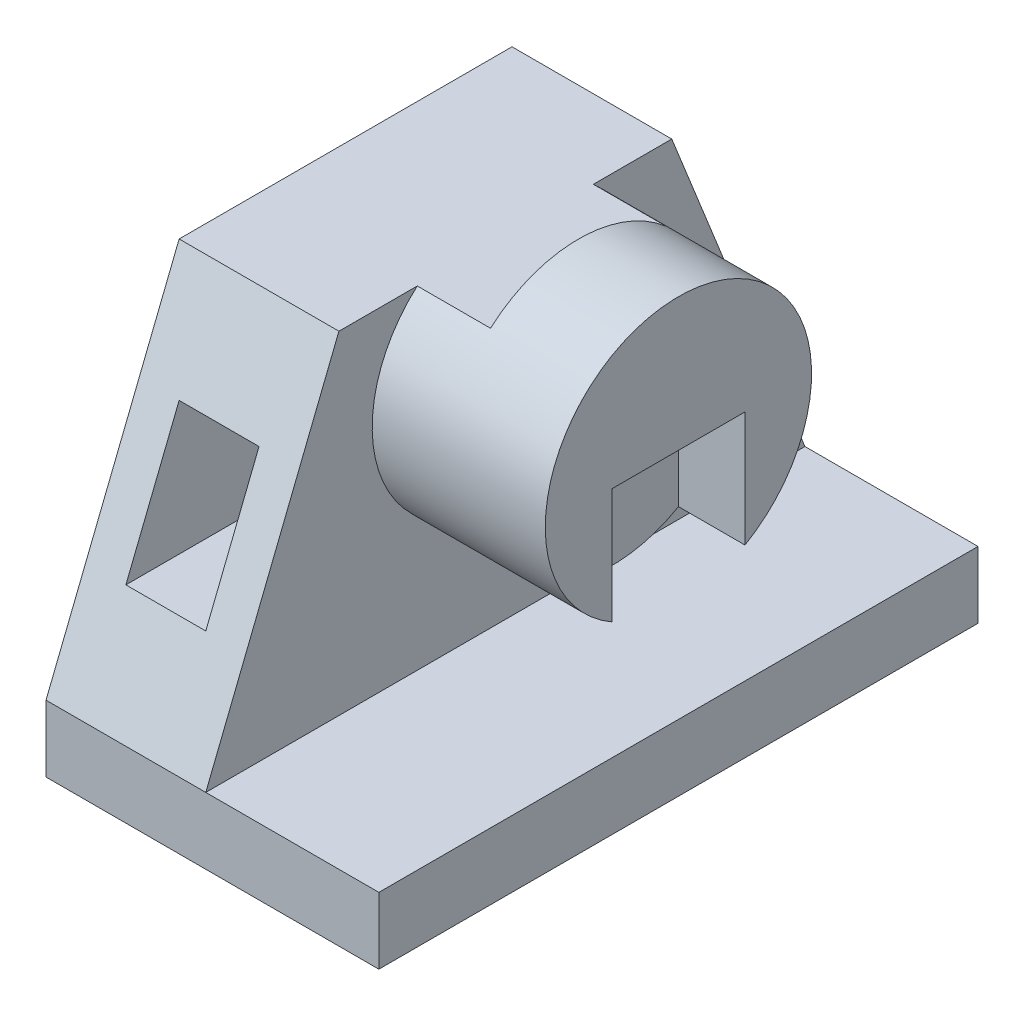
ISO-10303-21;
HEADER;
FILE_DESCRIPTION(('STEP AP214'),'2;1');
FILE_NAME('part.step','',(''),(''),'','','');
FILE_SCHEMA(('AUTOMOTIVE_DESIGN { 1 0 10303 214 1 1 1 1 }'));
ENDSEC;
DATA;
#1=APPLICATION_CONTEXT('core data for automotive mechanical design processes');
#2=APPLICATION_PROTOCOL_DEFINITION('international standard','automotive_design',2000,#1);
#3=PRODUCT_CONTEXT('',#1,'mechanical');
#4=PRODUCT('Part','Part','',(#3));
#5=PRODUCT_RELATED_PRODUCT_CATEGORY('part','',(#4));
#6=PRODUCT_DEFINITION_FORMATION('','',#4);
#7=PRODUCT_DEFINITION_CONTEXT('part definition',#1,'design');
#8=PRODUCT_DEFINITION('design','',#6,#7);
#9=PRODUCT_DEFINITION_SHAPE('','',#8);
#10=(LENGTH_UNIT() NAMED_UNIT(*) SI_UNIT(.MILLI.,.METRE.));
#11=(NAMED_UNIT(*) PLANE_ANGLE_UNIT() SI_UNIT($,.RADIAN.));
#12=(NAMED_UNIT(*) SI_UNIT($,.STERADIAN.) SOLID_ANGLE_UNIT());
#13=UNCERTAINTY_MEASURE_WITH_UNIT(LENGTH_MEASURE(1.E-05),#10,'distance_accuracy_value','');
#14=(GEOMETRIC_REPRESENTATION_CONTEXT(3) GLOBAL_UNCERTAINTY_ASSIGNED_CONTEXT((#13)) GLOBAL_UNIT_ASSIGNED_CONTEXT((#10,
#11,#12)) REPRESENTATION_CONTEXT('',''));
#15=CARTESIAN_POINT('',(0.,0.,0.));
#16=DIRECTION('',(0.,0.,1.));
#17=DIRECTION('',(1.,0.,0.));
#18=AXIS2_PLACEMENT_3D('',#15,#16,#17);
#19=CARTESIAN_POINT('',(-0.999999999999994,60.,-25.));
#20=DIRECTION('',(0.,0.371390676354104,-0.928476690885259));
#21=DIRECTION('',(0.,0.928476690885259,0.371390676354104));
#22=AXIS2_PLACEMENT_3D('',#19,#20,#21);
#23=PLANE('',#22);
#24=DIRECTION('',(0.,-0.928476690885259,-0.371390676354104));
#25=VECTOR('',#24,1.);
#26=CARTESIAN_POINT('',(-25.,60.,-25.));
#27=LINE('',#26,#25);
#28=CARTESIAN_POINT('',(-25.,60.,-25.));
#29=VERTEX_POINT('',#28);
#30=CARTESIAN_POINT('',(-25.,10.,-45.));
#31=VERTEX_POINT('',#30);
#32=EDGE_CURVE('E235',#29,#31,#27,.T.);
#33=ORIENTED_EDGE('',*,*,#32,.F.);
#34=DIRECTION('',(-1.,0.,0.));
#35=VECTOR('',#34,1.);
#36=CARTESIAN_POINT('',(-0.999999999999994,60.,-25.));
#37=LINE('',#36,#35);
#38=CARTESIAN_POINT('',(-0.999999999999994,60.,-25.));
#39=VERTEX_POINT('',#38);
#40=EDGE_CURVE('E251',#39,#29,#37,.T.);
#41=ORIENTED_EDGE('',*,*,#40,.F.);
#42=DIRECTION('',(0.,-0.928476690885259,-0.371390676354104));
#43=VECTOR('',#42,1.);
#44=CARTESIAN_POINT('',(-0.999999999999994,60.,-25.));
#45=LINE('',#44,#43);
#46=CARTESIAN_POINT('',(-0.999999999999994,10.,-45.));
#47=VERTEX_POINT('',#46);
#48=EDGE_CURVE('E239',#39,#47,#45,.T.);
#49=ORIENTED_EDGE('',*,*,#48,.T.);
#50=DIRECTION('',(-1.,0.,0.));
#51=VECTOR('',#50,1.);
#52=CARTESIAN_POINT('',(-0.999999999999994,10.,-45.));
#53=LINE('',#52,#51);
#54=EDGE_CURVE('E248',#47,#31,#53,.T.);
#55=ORIENTED_EDGE('',*,*,#54,.T.);
#56=EDGE_LOOP('',(#33,#41,#49,#55));
#57=FACE_BOUND('',#56,.T.);
#58=DIRECTION('',(-1.,0.,0.));
#59=VECTOR('',#58,1.);
#60=CARTESIAN_POINT('',(-0.999999999999994,45.,-31.));
#61=LINE('',#60,#59);
#62=CARTESIAN_POINT('',(-6.99999999999999,45.,-31.));
#63=VERTEX_POINT('',#62);
#64=CARTESIAN_POINT('',(-19.,45.,-31.));
#65=VERTEX_POINT('',#64);
#66=EDGE_CURVE('E225',#63,#65,#61,.T.);
#67=ORIENTED_EDGE('',*,*,#66,.T.);
#68=DIRECTION('',(0.,-0.928476690885259,-0.371390676354104));
#69=VECTOR('',#68,1.);
#70=CARTESIAN_POINT('',(-19.,60.,-25.));
#71=LINE('',#70,#69);
#72=CARTESIAN_POINT('',(-19.,25.,-39.));
#73=VERTEX_POINT('',#72);
#74=EDGE_CURVE('E223',#65,#73,#71,.T.);
#75=ORIENTED_EDGE('',*,*,#74,.T.);
#76=DIRECTION('',(1.,0.,0.));
#77=VECTOR('',#76,1.);
#78=CARTESIAN_POINT('',(-0.999999999999994,25.,-39.));
#79=LINE('',#78,#77);
#80=CARTESIAN_POINT('',(-6.99999999999999,25.,-39.));
#81=VERTEX_POINT('',#80);
#82=EDGE_CURVE('E216',#73,#81,#79,.T.);
#83=ORIENTED_EDGE('',*,*,#82,.T.);
#84=DIRECTION('',(0.,0.928476690885259,0.371390676354104));
#85=VECTOR('',#84,1.);
#86=CARTESIAN_POINT('',(-6.99999999999999,60.,-25.));
#87=LINE('',#86,#85);
#88=EDGE_CURVE('E218',#81,#63,#87,.T.);
#89=ORIENTED_EDGE('',*,*,#88,.T.);
#90=EDGE_LOOP('',(#67,#75,#83,#89));
#91=FACE_BOUND('',#90,.T.);
#92=ADVANCED_FACE('F39',(#57,#91),#23,.T.);
#93=CARTESIAN_POINT('',(-0.999999999999994,60.,25.));
#94=DIRECTION('',(0.,0.371390676354104,0.928476690885259));
#95=DIRECTION('',(0.,-0.928476690885259,0.371390676354104));
#96=AXIS2_PLACEMENT_3D('',#93,#94,#95);
#97=PLANE('',#96);
#98=DIRECTION('',(0.,0.928476690885259,-0.371390676354103));
#99=VECTOR('',#98,1.);
#100=CARTESIAN_POINT('',(-25.,60.,25.));
#101=LINE('',#100,#99);
#102=CARTESIAN_POINT('',(-25.,10.,45.));
#103=VERTEX_POINT('',#102);
#104=CARTESIAN_POINT('',(-25.,60.,25.));
#105=VERTEX_POINT('',#104);
#106=EDGE_CURVE('E229',#103,#105,#101,.T.);
#107=ORIENTED_EDGE('',*,*,#106,.F.);
#108=DIRECTION('',(1.,0.,0.));
#109=VECTOR('',#108,1.);
#110=CARTESIAN_POINT('',(-25.,10.,45.));
#111=LINE('',#110,#109);
#112=CARTESIAN_POINT('',(-0.999999999999994,10.,45.));
#113=VERTEX_POINT('',#112);
#114=EDGE_CURVE('E262',#103,#113,#111,.T.);
#115=ORIENTED_EDGE('',*,*,#114,.T.);
#116=DIRECTION('',(0.,0.928476690885259,-0.371390676354103));
#117=VECTOR('',#116,1.);
#118=CARTESIAN_POINT('',(-0.999999999999994,60.,25.));
#119=LINE('',#118,#117);
#120=CARTESIAN_POINT('',(-0.999999999999994,60.,25.));
#121=VERTEX_POINT('',#120);
#122=EDGE_CURVE('E234',#113,#121,#119,.T.);
#123=ORIENTED_EDGE('',*,*,#122,.T.);
#124=DIRECTION('',(-1.,0.,0.));
#125=VECTOR('',#124,1.);
#126=CARTESIAN_POINT('',(-0.999999999999994,60.,25.));
#127=LINE('',#126,#125);
#128=EDGE_CURVE('E242',#121,#105,#127,.T.);
#129=ORIENTED_EDGE('',*,*,#128,.T.);
#130=EDGE_LOOP('',(#107,#115,#123,#129));
#131=FACE_BOUND('',#130,.T.);
#132=DIRECTION('',(-1.,0.,0.));
#133=VECTOR('',#132,1.);
#134=CARTESIAN_POINT('',(-0.999999999999994,25.,39.));
#135=LINE('',#134,#133);
#136=CARTESIAN_POINT('',(-6.99999999999999,25.,39.));
#137=VERTEX_POINT('',#136);
#138=CARTESIAN_POINT('',(-19.,25.,39.));
#139=VERTEX_POINT('',#138);
#140=EDGE_CURVE('E287',#137,#139,#135,.T.);
#141=ORIENTED_EDGE('',*,*,#140,.T.);
#142=DIRECTION('',(0.,0.92847669088526,-0.371390676354104));
#143=VECTOR('',#142,1.);
#144=CARTESIAN_POINT('',(-19.,60.,25.));
#145=LINE('',#144,#143);
#146=CARTESIAN_POINT('',(-19.,45.,31.));
#147=VERTEX_POINT('',#146);
#148=EDGE_CURVE('E50',#139,#147,#145,.T.);
#149=ORIENTED_EDGE('',*,*,#148,.T.);
#150=DIRECTION('',(1.,0.,0.));
#151=VECTOR('',#150,1.);
#152=CARTESIAN_POINT('',(-0.999999999999994,45.,31.));
#153=LINE('',#152,#151);
#154=CARTESIAN_POINT('',(-7.,45.,31.));
#155=VERTEX_POINT('',#154);
#156=EDGE_CURVE('E295',#147,#155,#153,.T.);
#157=ORIENTED_EDGE('',*,*,#156,.T.);
#158=DIRECTION('',(0.,-0.92847669088526,0.371390676354104));
#159=VECTOR('',#158,1.);
#160=CARTESIAN_POINT('',(-7.,60.,25.));
#161=LINE('',#160,#159);
#162=EDGE_CURVE('E286',#155,#137,#161,.T.);
#163=ORIENTED_EDGE('',*,*,#162,.T.);
#164=EDGE_LOOP('',(#141,#149,#157,#163));
#165=FACE_BOUND('',#164,.T.);
#166=ADVANCED_FACE('F297',(#131,#165),#97,.T.);
#167=CARTESIAN_POINT('',(25.,10.,45.));
#168=DIRECTION('',(-1.,0.,0.));
#169=DIRECTION('',(0.,0.,1.));
#170=AXIS2_PLACEMENT_3D('',#167,#168,#169);
#171=PLANE('',#170);
#172=DIRECTION('',(0.,0.,-1.));
#173=VECTOR('',#172,1.);
#174=CARTESIAN_POINT('',(25.,0.,45.));
#175=LINE('',#174,#173);
#176=CARTESIAN_POINT('',(25.,0.,45.));
#177=VERTEX_POINT('',#176);
#178=CARTESIAN_POINT('',(25.,0.,-45.));
#179=VERTEX_POINT('',#178);
#180=EDGE_CURVE('E252',#177,#179,#175,.T.);
#181=ORIENTED_EDGE('',*,*,#180,.T.);
#182=DIRECTION('',(0.,-1.,0.));
#183=VECTOR('',#182,1.);
#184=CARTESIAN_POINT('',(25.,10.,-45.));
#185=LINE('',#184,#183);
#186=CARTESIAN_POINT('',(25.,10.,-45.));
#187=VERTEX_POINT('',#186);
#188=EDGE_CURVE('E284',#187,#179,#185,.T.);
#189=ORIENTED_EDGE('',*,*,#188,.F.);
#190=DIRECTION('',(0.,0.,-1.));
#191=VECTOR('',#190,1.);
#192=CARTESIAN_POINT('',(25.,10.,45.));
#193=LINE('',#192,#191);
#194=CARTESIAN_POINT('',(25.,10.,45.));
#195=VERTEX_POINT('',#194);
#196=EDGE_CURVE('E258',#195,#187,#193,.T.);
#197=ORIENTED_EDGE('',*,*,#196,.F.);
#198=DIRECTION('',(0.,-1.,0.));
#199=VECTOR('',#198,1.);
#200=CARTESIAN_POINT('',(25.,10.,45.));
#201=LINE('',#200,#199);
#202=EDGE_CURVE('E270',#195,#177,#201,.T.);
#203=ORIENTED_EDGE('',*,*,#202,.T.);
#204=EDGE_LOOP('',(#181,#189,#197,#203));
#205=FACE_BOUND('',#204,.T.);
#206=ADVANCED_FACE('F41',(#205),#171,.F.);
#207=CARTESIAN_POINT('',(-25.,10.,-45.));
#208=DIRECTION('',(0.,0.,1.));
#209=DIRECTION('',(1.,0.,0.));
#210=AXIS2_PLACEMENT_3D('',#207,#208,#209);
#211=PLANE('',#210);
#212=DIRECTION('',(-1.,0.,0.));
#213=VECTOR('',#212,1.);
#214=CARTESIAN_POINT('',(-25.,0.,-45.));
#215=LINE('',#214,#213);
#216=CARTESIAN_POINT('',(-25.,0.,-45.));
#217=VERTEX_POINT('',#216);
#218=EDGE_CURVE('E269',#179,#217,#215,.T.);
#219=ORIENTED_EDGE('',*,*,#218,.T.);
#220=DIRECTION('',(0.,-1.,0.));
#221=VECTOR('',#220,1.);
#222=CARTESIAN_POINT('',(-25.,10.,-45.));
#223=LINE('',#222,#221);
#224=EDGE_CURVE('E278',#31,#217,#223,.T.);
#225=ORIENTED_EDGE('',*,*,#224,.F.);
#226=ORIENTED_EDGE('',*,*,#54,.F.);
#227=DIRECTION('',(-1.,0.,0.));
#228=VECTOR('',#227,1.);
#229=CARTESIAN_POINT('',(-25.,10.,-45.));
#230=LINE('',#229,#228);
#231=EDGE_CURVE('E259',#187,#47,#230,.T.);
#232=ORIENTED_EDGE('',*,*,#231,.F.);
#233=ORIENTED_EDGE('',*,*,#188,.T.);
#234=EDGE_LOOP('',(#219,#225,#226,#232,#233));
#235=FACE_BOUND('',#234,.T.);
#236=ADVANCED_FACE('F347',(#235),#211,.F.);
#237=CARTESIAN_POINT('',(-25.,10.,45.));
#238=DIRECTION('',(1.,0.,0.));
#239=DIRECTION('',(0.,0.,-1.));
#240=AXIS2_PLACEMENT_3D('',#237,#238,#239);
#241=PLANE('',#240);
#242=DIRECTION('',(0.,0.,1.));
#243=VECTOR('',#242,1.);
#244=CARTESIAN_POINT('',(-25.,0.,45.));
#245=LINE('',#244,#243);
#246=CARTESIAN_POINT('',(-25.,0.,45.));
#247=VERTEX_POINT('',#246);
#248=EDGE_CURVE('E275',#217,#247,#245,.T.);
#249=ORIENTED_EDGE('',*,*,#248,.T.);
#250=DIRECTION('',(0.,-1.,0.));
#251=VECTOR('',#250,1.);
#252=CARTESIAN_POINT('',(-25.,10.,45.));
#253=LINE('',#252,#251);
#254=EDGE_CURVE('E280',#103,#247,#253,.T.);
#255=ORIENTED_EDGE('',*,*,#254,.F.);
#256=ORIENTED_EDGE('',*,*,#106,.T.);
#257=DIRECTION('',(0.,0.,-1.));
#258=VECTOR('',#257,1.);
#259=CARTESIAN_POINT('',(-25.,60.,-25.));
#260=LINE('',#259,#258);
#261=EDGE_CURVE('E245',#105,#29,#260,.T.);
#262=ORIENTED_EDGE('',*,*,#261,.T.);
#263=ORIENTED_EDGE('',*,*,#32,.T.);
#264=ORIENTED_EDGE('',*,*,#224,.T.);
#265=EDGE_LOOP('',(#249,#255,#256,#262,#263,#264));
#266=FACE_BOUND('',#265,.T.);
#267=ADVANCED_FACE('F345',(#266),#241,.F.);
#268=CARTESIAN_POINT('',(-25.,10.,45.));
#269=DIRECTION('',(0.,0.,-1.));
#270=DIRECTION('',(-1.,0.,0.));
#271=AXIS2_PLACEMENT_3D('',#268,#269,#270);
#272=PLANE('',#271);
#273=DIRECTION('',(1.,0.,0.));
#274=VECTOR('',#273,1.);
#275=CARTESIAN_POINT('',(-25.,0.,45.));
#276=LINE('',#275,#274);
#277=EDGE_CURVE('E257',#247,#177,#276,.T.);
#278=ORIENTED_EDGE('',*,*,#277,.T.);
#279=ORIENTED_EDGE('',*,*,#202,.F.);
#280=EDGE_CURVE('E263',#113,#195,#111,.T.);
#281=ORIENTED_EDGE('',*,*,#280,.F.);
#282=ORIENTED_EDGE('',*,*,#114,.F.);
#283=ORIENTED_EDGE('',*,*,#254,.T.);
#284=EDGE_LOOP('',(#278,#279,#281,#282,#283));
#285=FACE_BOUND('',#284,.T.);
#286=ADVANCED_FACE('F336',(#285),#272,.F.);
#287=CARTESIAN_POINT('',(0.,10.,0.));
#288=DIRECTION('',(0.,-1.,0.));
#289=DIRECTION('',(0.,0.,-1.));
#290=AXIS2_PLACEMENT_3D('',#287,#288,#289);
#291=PLANE('',#290);
#292=ORIENTED_EDGE('',*,*,#231,.T.);
#293=DIRECTION('',(0.,0.,1.));
#294=VECTOR('',#293,1.);
#295=CARTESIAN_POINT('',(-0.999999999999994,10.,-45.));
#296=LINE('',#295,#294);
#297=EDGE_CURVE('E228',#47,#113,#296,.T.);
#298=ORIENTED_EDGE('',*,*,#297,.T.);
#299=ORIENTED_EDGE('',*,*,#280,.T.);
#300=ORIENTED_EDGE('',*,*,#196,.T.);
#301=EDGE_LOOP('',(#292,#298,#299,#300));
#302=FACE_BOUND('',#301,.T.);
#303=ADVANCED_FACE('F331',(#302),#291,.F.);
#304=CARTESIAN_POINT('',(0.,0.,0.));
#305=DIRECTION('',(0.,-1.,0.));
#306=DIRECTION('',(0.,0.,-1.));
#307=AXIS2_PLACEMENT_3D('',#304,#305,#306);
#308=PLANE('',#307);
#309=ORIENTED_EDGE('',*,*,#180,.F.);
#310=ORIENTED_EDGE('',*,*,#277,.F.);
#311=ORIENTED_EDGE('',*,*,#248,.F.);
#312=ORIENTED_EDGE('',*,*,#218,.F.);
#313=EDGE_LOOP('',(#309,#310,#311,#312));
#314=FACE_BOUND('',#313,.T.);
#315=ADVANCED_FACE('F335',(#314),#308,.T.);
#316=CARTESIAN_POINT('',(-0.999999999999994,60.,-25.));
#317=DIRECTION('',(0.,1.,0.));
#318=DIRECTION('',(0.,0.,1.));
#319=AXIS2_PLACEMENT_3D('',#316,#317,#318);
#320=PLANE('',#319);
#321=ORIENTED_EDGE('',*,*,#261,.F.);
#322=ORIENTED_EDGE('',*,*,#128,.F.);
#323=DIRECTION('',(0.,0.,-1.));
#324=VECTOR('',#323,1.);
#325=CARTESIAN_POINT('',(-0.999999999999994,60.,-25.));
#326=LINE('',#325,#324);
#327=CARTESIAN_POINT('',(-0.999999999999994,60.,13.228756555323));
#328=VERTEX_POINT('',#327);
#329=EDGE_CURVE('E240',#121,#328,#326,.T.);
#330=ORIENTED_EDGE('',*,*,#329,.T.);
#331=DIRECTION('',(-1.,0.,0.));
#332=VECTOR('',#331,1.);
#333=CARTESIAN_POINT('',(10.,60.,13.228756555323));
#334=LINE('',#333,#332);
#335=CARTESIAN_POINT('',(10.,60.,13.228756555323));
#336=VERTEX_POINT('',#335);
#337=EDGE_CURVE('E172',#336,#328,#334,.T.);
#338=ORIENTED_EDGE('',*,*,#337,.F.);
#339=DIRECTION('',(0.,0.,1.));
#340=VECTOR('',#339,1.);
#341=CARTESIAN_POINT('',(10.,60.,-13.228756555323));
#342=LINE('',#341,#340);
#343=CARTESIAN_POINT('',(10.,60.,-13.228756555323));
#344=VERTEX_POINT('',#343);
#345=EDGE_CURVE('E165',#344,#336,#342,.T.);
#346=ORIENTED_EDGE('',*,*,#345,.F.);
#347=DIRECTION('',(-1.,0.,0.));
#348=VECTOR('',#347,1.);
#349=CARTESIAN_POINT('',(10.,60.,-13.228756555323));
#350=LINE('',#349,#348);
#351=CARTESIAN_POINT('',(-0.999999999999994,60.,-13.228756555323));
#352=VERTEX_POINT('',#351);
#353=EDGE_CURVE('E166',#344,#352,#350,.T.);
#354=ORIENTED_EDGE('',*,*,#353,.T.);
#355=EDGE_CURVE('E237',#352,#39,#326,.T.);
#356=ORIENTED_EDGE('',*,*,#355,.T.);
#357=ORIENTED_EDGE('',*,*,#40,.T.);
#358=EDGE_LOOP('',(#321,#322,#330,#338,#346,#354,#356,#357));
#359=FACE_BOUND('',#358,.T.);
#360=ADVANCED_FACE('F169',(#359),#320,.T.);
#361=CARTESIAN_POINT('',(-0.999999999999994,0.,0.));
#362=DIRECTION('',(1.,0.,0.));
#363=DIRECTION('',(0.,0.,-1.));
#364=AXIS2_PLACEMENT_3D('',#361,#362,#363);
#365=PLANE('',#364);
#366=ORIENTED_EDGE('',*,*,#355,.F.);
#367=CARTESIAN_POINT('',(-0.999999999999994,45.,0.));
#368=DIRECTION('',(1.,0.,0.));
#369=DIRECTION('',(0.,0.,-1.));
#370=AXIS2_PLACEMENT_3D('',#367,#368,#369);
#371=CIRCLE('',#370,20.);
#372=EDGE_CURVE('E11',#352,#328,#371,.F.);
#373=ORIENTED_EDGE('',*,*,#372,.T.);
#374=ORIENTED_EDGE('',*,*,#329,.F.);
#375=ORIENTED_EDGE('',*,*,#122,.F.);
#376=ORIENTED_EDGE('',*,*,#297,.F.);
#377=ORIENTED_EDGE('',*,*,#48,.F.);
#378=EDGE_LOOP('',(#366,#373,#374,#375,#376,#377));
#379=FACE_BOUND('',#378,.T.);
#380=ADVANCED_FACE('F328',(#379),#365,.T.);
#381=CARTESIAN_POINT('',(-19.,25.,-45.000012));
#382=DIRECTION('',(1.,0.,0.));
#383=DIRECTION('',(0.,0.,-1.));
#384=AXIS2_PLACEMENT_3D('',#381,#382,#383);
#385=PLANE('',#384);
#386=DIRECTION('',(0.,0.,1.));
#387=VECTOR('',#386,1.);
#388=CARTESIAN_POINT('',(-19.,45.,-45.000012));
#389=LINE('',#388,#387);
#390=EDGE_CURVE('E213',#65,#147,#389,.T.);
#391=ORIENTED_EDGE('',*,*,#390,.T.);
#392=ORIENTED_EDGE('',*,*,#148,.F.);
#393=DIRECTION('',(0.,0.,1.));
#394=VECTOR('',#393,1.);
#395=CARTESIAN_POINT('',(-19.,25.,-45.000012));
#396=LINE('',#395,#394);
#397=EDGE_CURVE('E210',#73,#139,#396,.T.);
#398=ORIENTED_EDGE('',*,*,#397,.F.);
#399=ORIENTED_EDGE('',*,*,#74,.F.);
#400=EDGE_LOOP('',(#391,#392,#398,#399));
#401=FACE_BOUND('',#400,.T.);
#402=ADVANCED_FACE('F300',(#401),#385,.T.);
#403=CARTESIAN_POINT('',(-6.99999999999999,45.,-45.000012));
#404=DIRECTION('',(0.,-1.,0.));
#405=DIRECTION('',(0.,0.,-1.));
#406=AXIS2_PLACEMENT_3D('',#403,#404,#405);
#407=PLANE('',#406);
#408=DIRECTION('',(0.,0.,1.));
#409=VECTOR('',#408,1.);
#410=CARTESIAN_POINT('',(-6.99999999999999,45.,-45.000012));
#411=LINE('',#410,#409);
#412=EDGE_CURVE('E209',#63,#155,#411,.T.);
#413=ORIENTED_EDGE('',*,*,#412,.T.);
#414=ORIENTED_EDGE('',*,*,#156,.F.);
#415=ORIENTED_EDGE('',*,*,#390,.F.);
#416=ORIENTED_EDGE('',*,*,#66,.F.);
#417=EDGE_LOOP('',(#413,#414,#415,#416));
#418=FACE_BOUND('',#417,.T.);
#419=ADVANCED_FACE('F305',(#418),#407,.T.);
#420=CARTESIAN_POINT('',(-6.99999999999999,25.,-45.000012));
#421=DIRECTION('',(-1.,0.,0.));
#422=DIRECTION('',(0.,0.,1.));
#423=AXIS2_PLACEMENT_3D('',#420,#421,#422);
#424=PLANE('',#423);
#425=DIRECTION('',(0.,0.,1.));
#426=VECTOR('',#425,1.);
#427=CARTESIAN_POINT('',(-6.99999999999999,25.,-45.000012));
#428=LINE('',#427,#426);
#429=EDGE_CURVE('E62',#81,#137,#428,.T.);
#430=ORIENTED_EDGE('',*,*,#429,.T.);
#431=ORIENTED_EDGE('',*,*,#162,.F.);
#432=ORIENTED_EDGE('',*,*,#412,.F.);
#433=ORIENTED_EDGE('',*,*,#88,.F.);
#434=EDGE_LOOP('',(#430,#431,#432,#433));
#435=FACE_BOUND('',#434,.T.);
#436=ADVANCED_FACE('F307',(#435),#424,.T.);
#437=CARTESIAN_POINT('',(-6.99999999999999,25.,-45.000012));
#438=DIRECTION('',(0.,1.,0.));
#439=DIRECTION('',(0.,0.,1.));
#440=AXIS2_PLACEMENT_3D('',#437,#438,#439);
#441=PLANE('',#440);
#442=ORIENTED_EDGE('',*,*,#397,.T.);
#443=ORIENTED_EDGE('',*,*,#140,.F.);
#444=ORIENTED_EDGE('',*,*,#429,.F.);
#445=ORIENTED_EDGE('',*,*,#82,.F.);
#446=EDGE_LOOP('',(#442,#443,#444,#445));
#447=FACE_BOUND('',#446,.T.);
#448=ADVANCED_FACE('F310',(#447),#441,.T.);
#449=CARTESIAN_POINT('',(25.,45.,0.));
#450=DIRECTION('',(-1.,0.,0.));
#451=DIRECTION('',(0.,0.,1.));
#452=AXIS2_PLACEMENT_3D('',#449,#450,#451);
#453=CYLINDRICAL_SURFACE('',#452,20.);
#454=CARTESIAN_POINT('',(15.,45.,0.));
#455=DIRECTION('',(1.,0.,0.));
#456=DIRECTION('',(0.,0.,-1.));
#457=AXIS2_PLACEMENT_3D('',#454,#455,#456);
#458=CIRCLE('',#457,20.);
#459=CARTESIAN_POINT('',(15.,27.6794919243112,9.99999999999999));
#460=VERTEX_POINT('',#459);
#461=CARTESIAN_POINT('',(15.,27.6794919243112,-10.));
#462=VERTEX_POINT('',#461);
#463=EDGE_CURVE('E181',#460,#462,#458,.T.);
#464=ORIENTED_EDGE('',*,*,#463,.F.);
#465=DIRECTION('',(1.,0.,0.));
#466=VECTOR('',#465,1.);
#467=CARTESIAN_POINT('',(15.,27.6794919243112,9.99999999999999));
#468=LINE('',#467,#466);
#469=CARTESIAN_POINT('',(25.,27.6794919243112,9.99999999999999));
#470=VERTEX_POINT('',#469);
#471=EDGE_CURVE('E192',#460,#470,#468,.T.);
#472=ORIENTED_EDGE('',*,*,#471,.T.);
#473=CARTESIAN_POINT('',(25.,45.,0.));
#474=DIRECTION('',(1.,0.,0.));
#475=DIRECTION('',(0.,0.,-1.));
#476=AXIS2_PLACEMENT_3D('',#473,#474,#475);
#477=CIRCLE('',#476,20.);
#478=CARTESIAN_POINT('',(25.,27.6794919243112,-10.));
#479=VERTEX_POINT('',#478);
#480=EDGE_CURVE('E200',#479,#470,#477,.T.);
#481=ORIENTED_EDGE('',*,*,#480,.F.);
#482=DIRECTION('',(1.,0.,0.));
#483=VECTOR('',#482,1.);
#484=CARTESIAN_POINT('',(15.,27.6794919243112,-10.));
#485=LINE('',#484,#483);
#486=EDGE_CURVE('E53',#462,#479,#485,.T.);
#487=ORIENTED_EDGE('',*,*,#486,.F.);
#488=EDGE_LOOP('',(#464,#472,#481,#487));
#489=FACE_BOUND('',#488,.T.);
#490=CARTESIAN_POINT('',(10.,45.,0.));
#491=DIRECTION('',(-1.,0.,0.));
#492=DIRECTION('',(0.,0.,1.));
#493=AXIS2_PLACEMENT_3D('',#490,#491,#492);
#494=CIRCLE('',#493,20.);
#495=EDGE_CURVE('E157',#336,#344,#494,.T.);
#496=ORIENTED_EDGE('',*,*,#495,.F.);
#497=ORIENTED_EDGE('',*,*,#337,.T.);
#498=ORIENTED_EDGE('',*,*,#372,.F.);
#499=ORIENTED_EDGE('',*,*,#353,.F.);
#500=EDGE_LOOP('',(#496,#497,#498,#499));
#501=FACE_BOUND('',#500,.T.);
#502=ADVANCED_FACE('F173',(#489,#501),#453,.T.);
#503=CARTESIAN_POINT('',(25.,45.,0.));
#504=DIRECTION('',(1.,0.,0.));
#505=DIRECTION('',(0.,0.,-1.));
#506=AXIS2_PLACEMENT_3D('',#503,#504,#505);
#507=PLANE('',#506);
#508=DIRECTION('',(0.,-1.,0.));
#509=VECTOR('',#508,1.);
#510=CARTESIAN_POINT('',(25.,45.,10.));
#511=LINE('',#510,#509);
#512=CARTESIAN_POINT('',(25.,45.,10.));
#513=VERTEX_POINT('',#512);
#514=EDGE_CURVE('E179',#513,#470,#511,.T.);
#515=ORIENTED_EDGE('',*,*,#514,.F.);
#516=DIRECTION('',(0.,0.,-1.));
#517=VECTOR('',#516,1.);
#518=CARTESIAN_POINT('',(25.,45.,10.));
#519=LINE('',#518,#517);
#520=CARTESIAN_POINT('',(25.,45.,-10.));
#521=VERTEX_POINT('',#520);
#522=EDGE_CURVE('E184',#513,#521,#519,.T.);
#523=ORIENTED_EDGE('',*,*,#522,.T.);
#524=DIRECTION('',(0.,-1.,0.));
#525=VECTOR('',#524,1.);
#526=CARTESIAN_POINT('',(25.,45.,-10.));
#527=LINE('',#526,#525);
#528=EDGE_CURVE('E195',#521,#479,#527,.T.);
#529=ORIENTED_EDGE('',*,*,#528,.T.);
#530=ORIENTED_EDGE('',*,*,#480,.T.);
#531=EDGE_LOOP('',(#515,#523,#529,#530));
#532=FACE_BOUND('',#531,.T.);
#533=ADVANCED_FACE('F404',(#532),#507,.T.);
#534=CARTESIAN_POINT('',(15.,45.,10.));
#535=DIRECTION('',(0.,0.,1.));
#536=DIRECTION('',(1.,0.,0.));
#537=AXIS2_PLACEMENT_3D('',#534,#535,#536);
#538=PLANE('',#537);
#539=ORIENTED_EDGE('',*,*,#514,.T.);
#540=ORIENTED_EDGE('',*,*,#471,.F.);
#541=DIRECTION('',(0.,-1.,0.));
#542=VECTOR('',#541,1.);
#543=CARTESIAN_POINT('',(15.,45.,10.));
#544=LINE('',#543,#542);
#545=CARTESIAN_POINT('',(15.,45.,10.));
#546=VERTEX_POINT('',#545);
#547=EDGE_CURVE('E178',#546,#460,#544,.T.);
#548=ORIENTED_EDGE('',*,*,#547,.F.);
#549=DIRECTION('',(1.,0.,0.));
#550=VECTOR('',#549,1.);
#551=CARTESIAN_POINT('',(15.,45.,10.));
#552=LINE('',#551,#550);
#553=EDGE_CURVE('E197',#546,#513,#552,.T.);
#554=ORIENTED_EDGE('',*,*,#553,.T.);
#555=EDGE_LOOP('',(#539,#540,#548,#554));
#556=FACE_BOUND('',#555,.T.);
#557=ADVANCED_FACE('F411',(#556),#538,.F.);
#558=CARTESIAN_POINT('',(15.,45.,10.));
#559=DIRECTION('',(0.,-1.,0.));
#560=DIRECTION('',(0.,0.,-1.));
#561=AXIS2_PLACEMENT_3D('',#558,#559,#560);
#562=PLANE('',#561);
#563=ORIENTED_EDGE('',*,*,#522,.F.);
#564=ORIENTED_EDGE('',*,*,#553,.F.);
#565=DIRECTION('',(0.,0.,-1.));
#566=VECTOR('',#565,1.);
#567=CARTESIAN_POINT('',(15.,45.,10.));
#568=LINE('',#567,#566);
#569=CARTESIAN_POINT('',(15.,45.,-10.));
#570=VERTEX_POINT('',#569);
#571=EDGE_CURVE('E188',#546,#570,#568,.T.);
#572=ORIENTED_EDGE('',*,*,#571,.T.);
#573=DIRECTION('',(1.,0.,0.));
#574=VECTOR('',#573,1.);
#575=CARTESIAN_POINT('',(15.,45.,-10.));
#576=LINE('',#575,#574);
#577=EDGE_CURVE('E199',#570,#521,#576,.T.);
#578=ORIENTED_EDGE('',*,*,#577,.T.);
#579=EDGE_LOOP('',(#563,#564,#572,#578));
#580=FACE_BOUND('',#579,.T.);
#581=ADVANCED_FACE('F424',(#580),#562,.T.);
#582=CARTESIAN_POINT('',(15.,45.,-10.));
#583=DIRECTION('',(0.,0.,1.));
#584=DIRECTION('',(0.,-1.,0.));
#585=AXIS2_PLACEMENT_3D('',#582,#583,#584);
#586=PLANE('',#585);
#587=ORIENTED_EDGE('',*,*,#528,.F.);
#588=ORIENTED_EDGE('',*,*,#577,.F.);
#589=DIRECTION('',(0.,-1.,0.));
#590=VECTOR('',#589,1.);
#591=CARTESIAN_POINT('',(15.,45.,-10.));
#592=LINE('',#591,#590);
#593=EDGE_CURVE('E187',#570,#462,#592,.T.);
#594=ORIENTED_EDGE('',*,*,#593,.T.);
#595=ORIENTED_EDGE('',*,*,#486,.T.);
#596=EDGE_LOOP('',(#587,#588,#594,#595));
#597=FACE_BOUND('',#596,.T.);
#598=ADVANCED_FACE('F432',(#597),#586,.T.);
#599=CARTESIAN_POINT('',(15.,45.,0.));
#600=DIRECTION('',(1.,0.,0.));
#601=DIRECTION('',(0.,0.,-1.));
#602=AXIS2_PLACEMENT_3D('',#599,#600,#601);
#603=PLANE('',#602);
#604=ORIENTED_EDGE('',*,*,#547,.T.);
#605=ORIENTED_EDGE('',*,*,#463,.T.);
#606=ORIENTED_EDGE('',*,*,#593,.F.);
#607=ORIENTED_EDGE('',*,*,#571,.F.);
#608=EDGE_LOOP('',(#604,#605,#606,#607));
#609=FACE_BOUND('',#608,.T.);
#610=ADVANCED_FACE('F441',(#609),#603,.T.);
#611=CARTESIAN_POINT('',(10.,45.,0.));
#612=DIRECTION('',(-1.,0.,0.));
#613=DIRECTION('',(0.,0.,1.));
#614=AXIS2_PLACEMENT_3D('',#611,#612,#613);
#615=PLANE('',#614);
#616=ORIENTED_EDGE('',*,*,#495,.T.);
#617=ORIENTED_EDGE('',*,*,#345,.T.);
#618=EDGE_LOOP('',(#616,#617));
#619=FACE_BOUND('',#618,.T.);
#620=ADVANCED_FACE('F161',(#619),#615,.T.);
#621=CLOSED_SHELL('',(#92,#166,#206,#236,#267,#286,#303,#315,#360,#380,#402,#419,#436,#448,#502,
#533,#557,#581,#598,#610,#620));
#622=MANIFOLD_SOLID_BREP('B2',#621);
#623=ADVANCED_BREP_SHAPE_REPRESENTATION('',(#18,#622),#14);
#624=SHAPE_DEFINITION_REPRESENTATION(#9,#623);
ENDSEC;
END-ISO-10303-21;
